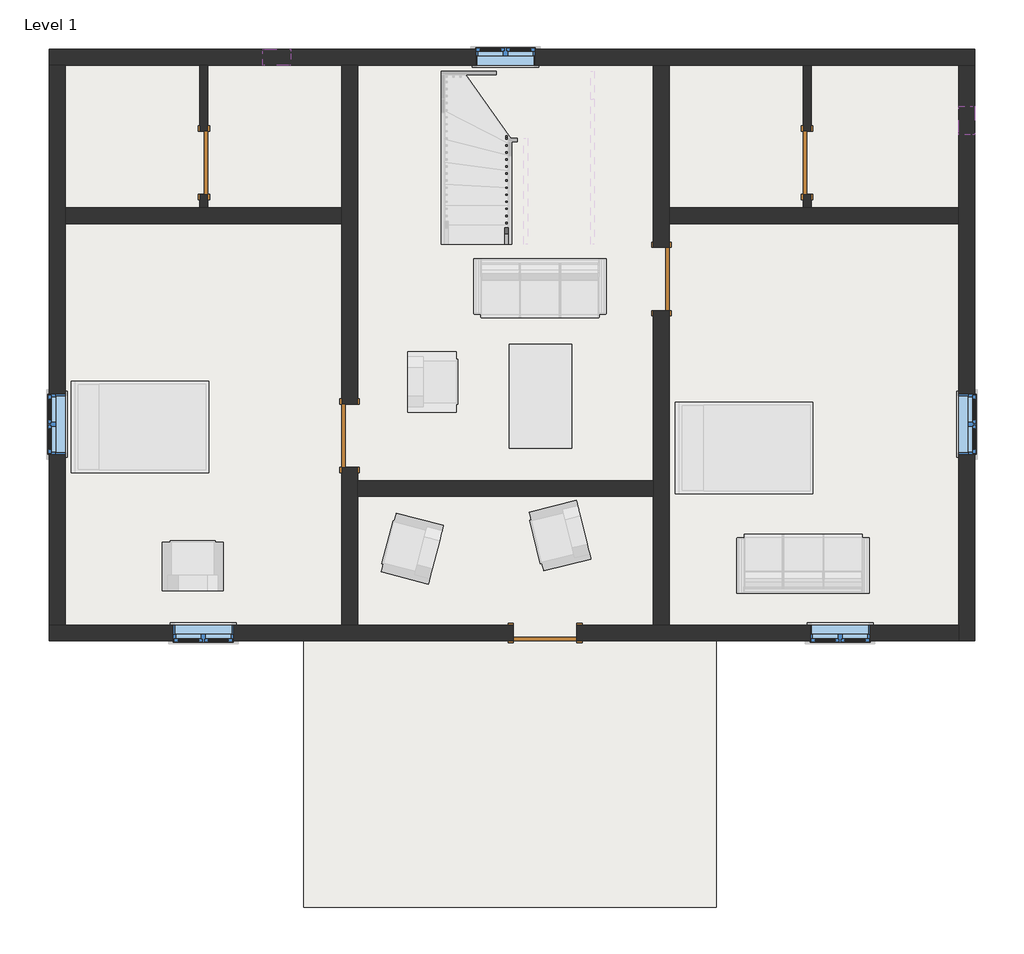
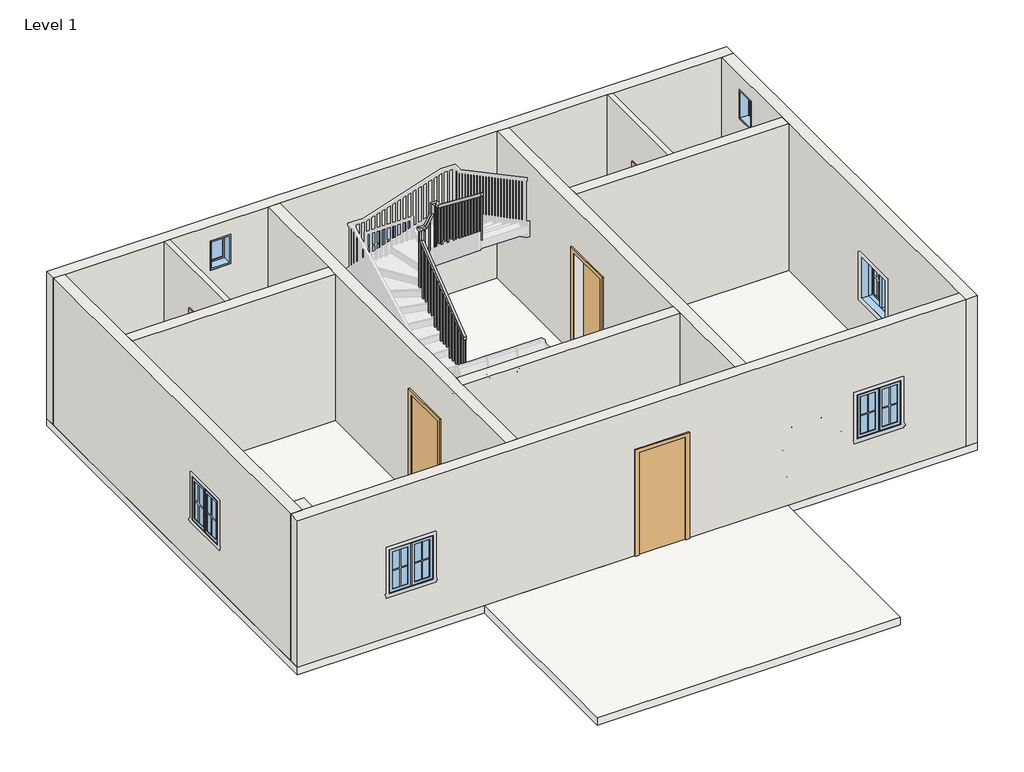
# One storey, part 1 of 2: 11 walls, 7 windows, 5 doors, 2 slabs, 1 railing.
"""IFC4 building model written with IfcOpenShell, lengths in millimetres."""

from ifc_helpers import new_model, si_unit, frame, origin, origin_with_axes, place, context, project, spatial, polyline, outline, extrude, faceted_brep, transform, mapped, element, save
from components import door_e5f9f3c4, door_a90ba1ad, door_305aa2a5, door_0ca8825f, window_aa618e30, window_339605e1

model = new_model("IFC4")

# Units and contexts
model_context = context("Model", 3, world=origin())
ifc_project = project(units=[si_unit("LENGTHUNIT", "METRE", prefix="MILLI")], contexts=[model_context])

# Site, building, storey
site = spatial("IfcSite", under=ifc_project)
building = spatial("IfcBuilding", under=site)
storey = spatial("IfcBuildingStorey", under=building, Name="Level 1", Elevation=0.0)

# Doors
placement = place(None, origin())
door_shape = door_e5f9f3c4(model_context)
element("IfcDoor", 1, ObjectType="Single-Flush : 36\" x 84\"", at=placement, inside=storey, context=model_context, shape_type="MappedRepresentation", body=[
    mapped(door_shape, transform((-5102.9390964, 4820.103532, 0.0), x_axis=(0.0, -1.0, 0.0), y_axis=(1.0, 0.0, 0.0), z_axis=(0.0, 0.0, 1.0))),
])
door_2_shape = door_a90ba1ad(model_context)
element("IfcDoor", 2, ObjectType="Single-Flush : 36\" x 84\"", at=placement, inside=storey, context=model_context, shape_type="MappedRepresentation", body=[
    mapped(door_2_shape, transform((-3001.0890964, 883.103532, 0.0), x_axis=(0.0, -1.0, 0.0), y_axis=(1.0, 0.0, 0.0), z_axis=(0.0, 0.0, 1.0))),
])
element("IfcDoor", 3, ObjectType="Single-Flush : 36\" x 84\"", at=placement, inside=storey, context=model_context, shape_type="MappedRepresentation", body=[
    mapped(door_2_shape, transform((1494.7109036, 3143.703532, 0.0), x_axis=(0.0, 1.0, 0.0), y_axis=(-1.0, 0.0, 0.0), z_axis=(0.0, 0.0, 1.0))),
])
door_3_shape = door_305aa2a5(model_context)
element("IfcDoor", 4, ObjectType="Single-Flush : 36\" x 84\"", at=placement, inside=storey, context=model_context, shape_type="MappedRepresentation", body=[
    mapped(door_3_shape, transform((3596.5609036, 4820.103532, 0.0), x_axis=(0.0, -1.0, 0.0), y_axis=(1.0, 0.0, 0.0), z_axis=(0.0, 0.0, 1.0))),
])
door_4_shape = door_0ca8825f(model_context)
element("IfcDoor", 5, ObjectType="Single-Flush : 36\" x 84\"", at=placement, inside=storey, context=model_context, shape_type="MappedRepresentation", body=[
    mapped(door_4_shape, transform((-181.6890964, -1961.696468, 0.0), x_axis=(-1.0, 0.0, 0.0), y_axis=(0.0, -1.0, 0.0), z_axis=(0.0, 0.0, 1.0))),
])

# Railing
element("IfcRailing", 6, ObjectType="Handrail - Rectangular", at=placement, inside=storey, context=model_context, shape_type="SolidModel", body=[
    faceted_brep([(-765.8890964, 3647.9718401, 1083.7333333), (-765.8890964, 3647.9718401, 1019.4000346), (-715.0890964, 3647.9718401, 1019.4000346), (-715.0890964, 3647.9718401, 1083.7333333), (-765.8890964, 5099.503532, 2211.6191036), (-765.8890964, 5150.303532, 2186.7590024), (-715.0890964, 5150.303532, 2186.7590024), (-715.0890964, 5099.503532, 2211.6191036), (-765.8890964, 5099.503532, 2414.6281882), (-765.8890964, 5150.303532, 2363.8281882), (-715.0890964, 5150.303532, 2363.8281882), (-715.0890964, 5099.503532, 2414.6281882), (-765.8890964, 5226.503532, 2414.6281882), (-765.8890964, 5226.503532, 2363.8281882), (-715.0890964, 5175.703532, 2363.8281882), (-715.0890964, 5175.703532, 2414.6281882), (-638.8890964, 5226.503532, 2414.6281882), (-609.7677625, 5226.503532, 2363.8281882), (-609.7677625, 5175.703532, 2363.8281882), (-638.8890964, 5175.703532, 2414.6281882), (-511.8890964, 5226.503532, 2631.5051451), (-461.0890964, 5226.503532, 2617.7256424), (-461.0890964, 5175.703532, 2617.7256424), (-511.8890964, 5175.703532, 2631.5051451), (-511.8890964, 5226.503532, 2834.5142297), (-461.0890964, 5226.503532, 2783.7142297), (-461.0890964, 5175.703532, 2783.7142297), (-511.8890964, 5175.703532, 2834.5142297), (-384.8890964, 5226.503532, 2834.5142297), (-384.8890964, 5226.503532, 2783.7142297), (-435.6890964, 5175.703532, 2783.7142297), (-435.6890964, 5175.703532, 2834.5142297), (-384.8890964, 5099.503532, 2834.5142297), (-384.8890964, 5082.086864, 2783.7142297), (-435.6890964, 5082.086864, 2783.7142297), (-435.6890964, 5099.503532, 2834.5142297), (-384.8890964, 3647.9718401, 3962.4), (-435.6890964, 3647.9718401, 3962.4), (-435.6890964, 3647.9718401, 3898.0667013), (-384.8890964, 3647.9718401, 3898.0667013)], [[[0, 1, 2, 3]], [[1, 0, 4, 5]], [[2, 1, 5, 6]], [[3, 2, 6, 7]], [[0, 3, 7, 4]], [[5, 4, 8, 9]], [[6, 5, 9, 10]], [[7, 6, 10, 11]], [[4, 7, 11, 8]], [[9, 8, 12, 13]], [[10, 9, 13, 14]], [[11, 10, 14, 15]], [[8, 11, 15, 12]], [[13, 12, 16, 17]], [[14, 13, 17, 18]], [[15, 14, 18, 19]], [[12, 15, 19, 16]], [[17, 16, 20, 21]], [[18, 17, 21, 22]], [[19, 18, 22, 23]], [[16, 19, 23, 20]], [[21, 20, 24, 25]], [[22, 21, 25, 26]], [[23, 22, 26, 27]], [[20, 23, 27, 24]], [[25, 24, 28, 29]], [[26, 25, 29, 30]], [[27, 26, 30, 31]], [[24, 27, 31, 28]], [[29, 28, 32, 33]], [[30, 29, 33, 34]], [[31, 30, 34, 35]], [[28, 31, 35, 32]], [[36, 37, 38, 39]], [[33, 32, 36, 39]], [[34, 33, 39, 38]], [[35, 34, 38, 37]], [[32, 35, 37, 36]]]),
    extrude(outline(polyline([(3667.578532, 3882.8316852), (3686.628532, 3868.0292361), (3686.628532, 2878.6666667), (3667.578532, 2878.6666667), (3667.578532, 3882.8316852)])), frame((-419.8140964, 0.0, 0.0), z_axis=(1.0, 0.0, 0.0), x_axis=(0.0, 1.0, 0.0)), (0.0, 0.0, 1.0), 19.05),
    extrude(outline(polyline([(3769.178532, 3803.8852902), (3788.228532, 3789.0828411), (3788.228532, 2878.6666667), (3769.178532, 2878.6666667), (3769.178532, 3803.8852902)])), frame((-419.8140964, 0.0, 0.0), z_axis=(1.0, 0.0, 0.0), x_axis=(0.0, 1.0, 0.0)), (0.0, 0.0, 1.0), 19.05),
    extrude(outline(polyline([(3870.778532, 3724.9388952), (3889.828532, 3710.1364462), (3889.828532, 2878.6666667), (3870.778532, 2878.6666667), (3870.778532, 3724.9388952)])), frame((-419.8140964, 0.0, 0.0), z_axis=(1.0, 0.0, 0.0), x_axis=(0.0, 1.0, 0.0)), (0.0, 0.0, 1.0), 19.05),
    extrude(outline(polyline([(3972.378532, 3645.9925003), (3991.428532, 3631.1900512), (3991.428532, 2709.3333333), (3972.378532, 2709.3333333), (3972.378532, 3645.9925003)])), frame((-419.8140964, 0.0, 0.0), z_axis=(1.0, 0.0, 0.0), x_axis=(0.0, 1.0, 0.0)), (0.0, 0.0, 1.0), 19.05),
    extrude(outline(polyline([(4073.978532, 3567.0461053), (4093.028532, 3552.2436562), (4093.028532, 2709.3333333), (4073.978532, 2709.3333333), (4073.978532, 3567.0461053)])), frame((-419.8140964, 0.0, 0.0), z_axis=(1.0, 0.0, 0.0), x_axis=(0.0, 1.0, 0.0)), (0.0, 0.0, 1.0), 19.05),
    extrude(outline(polyline([(4175.578532, 3488.0997103), (4194.628532, 3473.2972613), (4194.628532, 2709.3333333), (4175.578532, 2709.3333333), (4175.578532, 3488.0997103)])), frame((-419.8140964, 0.0, 0.0), z_axis=(1.0, 0.0, 0.0), x_axis=(0.0, 1.0, 0.0)), (0.0, 0.0, 1.0), 19.05),
    extrude(outline(polyline([(4277.178532, 3409.1533154), (4296.228532, 3394.3508663), (4296.228532, 2540.0), (4277.178532, 2540.0), (4277.178532, 3409.1533154)])), frame((-419.8140964, 0.0, 0.0), z_axis=(1.0, 0.0, 0.0), x_axis=(0.0, 1.0, 0.0)), (0.0, 0.0, 1.0), 19.05),
    extrude(outline(polyline([(4378.778532, 3330.2069204), (4397.828532, 3315.4044713), (4397.828532, 2540.0), (4378.778532, 2540.0), (4378.778532, 3330.2069204)])), frame((-419.8140964, 0.0, 0.0), z_axis=(1.0, 0.0, 0.0), x_axis=(0.0, 1.0, 0.0)), (0.0, 0.0, 1.0), 19.05),
    extrude(outline(polyline([(4480.378532, 3251.2605254), (4499.428532, 3236.4580764), (4499.428532, 2370.6666667), (4480.378532, 2370.6666667), (4480.378532, 3251.2605254)])), frame((-419.8140964, 0.0, 0.0), z_axis=(1.0, 0.0, 0.0), x_axis=(0.0, 1.0, 0.0)), (0.0, 0.0, 1.0), 19.05),
    extrude(outline(polyline([(4581.978532, 3172.3141304), (4601.028532, 3157.5116814), (4601.028532, 2370.6666667), (4581.978532, 2370.6666667), (4581.978532, 3172.3141304)])), frame((-419.8140964, 0.0, 0.0), z_axis=(1.0, 0.0, 0.0), x_axis=(0.0, 1.0, 0.0)), (0.0, 0.0, 1.0), 19.05),
    extrude(outline(polyline([(4683.578532, 3093.3677355), (4702.628532, 3078.5652864), (4702.628532, 2370.6666667), (4683.578532, 2370.6666667), (4683.578532, 3093.3677355)])), frame((-419.8140964, 0.0, 0.0), z_axis=(1.0, 0.0, 0.0), x_axis=(0.0, 1.0, 0.0)), (0.0, 0.0, 1.0), 19.05),
    extrude(outline(polyline([(4785.178532, 3014.4213405), (4804.228532, 2999.6188914), (4804.228532, 2201.3333333), (4785.178532, 2201.3333333), (4785.178532, 3014.4213405)])), frame((-419.8140964, 0.0, 0.0), z_axis=(1.0, 0.0, 0.0), x_axis=(0.0, 1.0, 0.0)), (0.0, 0.0, 1.0), 19.05),
    extrude(outline(polyline([(4886.778532, 2935.4749455), (4905.828532, 2920.6724965), (4905.828532, 2201.3333333), (4886.778532, 2201.3333333), (4886.778532, 2935.4749455)])), frame((-419.8140964, 0.0, 0.0), z_axis=(1.0, 0.0, 0.0), x_axis=(0.0, 1.0, 0.0)), (0.0, 0.0, 1.0), 19.05),
    extrude(outline(polyline([(4988.378532, 2856.5285506), (5007.428532, 2841.7261015), (5007.428532, 2032.0), (4988.378532, 2032.0), (4988.378532, 2856.5285506)])), frame((-419.8140964, 0.0, 0.0), z_axis=(1.0, 0.0, 0.0), x_axis=(0.0, 1.0, 0.0)), (0.0, 0.0, 1.0), 19.05),
    extrude(outline(polyline([(5089.978532, 2777.5821556), (5109.028532, 2762.7797065), (5109.028532, 2032.0), (5089.978532, 2032.0), (5089.978532, 2777.5821556)])), frame((-419.8140964, 0.0, 0.0), z_axis=(1.0, 0.0, 0.0), x_axis=(0.0, 1.0, 0.0)), (0.0, 0.0, 1.0), 19.05),
    extrude(outline(polyline([(-445.2140964, 5191.578532), (-445.2140964, 5210.628532), (-426.1640964, 5210.628532), (-426.1640964, 5191.578532), (-445.2140964, 5191.578532)])), frame((0.0, 0.0, 1693.3333333), z_axis=(0.0, 0.0, 1.0), x_axis=(1.0, 0.0, 0.0)), (0.0, 0.0, 1.0), 1090.3808964),
    extrude(outline(polyline([(2503.86524, -527.7640964), (2471.3336964, -546.8140964), (1524.0, -546.8140964), (1524.0, -527.7640964), (2503.86524, -527.7640964)])), frame((0.0, 5191.578532, 0.0), z_axis=(0.0, 1.0, 0.0), x_axis=(0.0, 0.0, 1.0)), (0.0, 0.0, 1.0), 19.05),
    extrude(outline(polyline([(2330.3636744, -629.3640964), (2297.8321309, -648.4140964), (1354.6666667, -648.4140964), (1354.6666667, -629.3640964), (2330.3636744, -629.3640964)])), frame((0.0, 5191.578532, 0.0), z_axis=(0.0, 1.0, 0.0), x_axis=(0.0, 0.0, 1.0)), (0.0, 0.0, 1.0), 19.05),
    extrude(outline(polyline([(-730.9640964, 5162.4468401), (-750.0140964, 5162.4468401), (-750.0140964, 5181.4968401), (-730.9640964, 5181.4968401), (-730.9640964, 5162.4468401)])), frame((0.0, 0.0, 1185.3333333), z_axis=(0.0, 0.0, 1.0), x_axis=(1.0, 0.0, 0.0)), (0.0, 0.0, 1.0), 1178.4948549),
    extrude(outline(polyline([(5060.8468401, 2117.2483397), (5079.8968401, 2132.0507888), (5079.8968401, 1016.0), (5060.8468401, 1016.0), (5060.8468401, 2117.2483397)])), frame((-750.0140964, 0.0, 0.0), z_axis=(1.0, 0.0, 0.0), x_axis=(0.0, 1.0, 0.0)), (0.0, 0.0, 1.0), 19.05),
    extrude(outline(polyline([(4959.2468401, 2038.3019447), (4978.2968401, 2053.1043938), (4978.2968401, 1016.0), (4959.2468401, 1016.0), (4959.2468401, 2038.3019447)])), frame((-750.0140964, 0.0, 0.0), z_axis=(1.0, 0.0, 0.0), x_axis=(0.0, 1.0, 0.0)), (0.0, 0.0, 1.0), 19.05),
    extrude(outline(polyline([(4857.6468401, 1959.3555498), (4876.6968401, 1974.1579988), (4876.6968401, 846.6666667), (4857.6468401, 846.6666667), (4857.6468401, 1959.3555498)])), frame((-750.0140964, 0.0, 0.0), z_axis=(1.0, 0.0, 0.0), x_axis=(0.0, 1.0, 0.0)), (0.0, 0.0, 1.0), 19.05),
    extrude(outline(polyline([(4756.0468401, 1880.4091548), (4775.0968401, 1895.2116039), (4775.0968401, 846.6666667), (4756.0468401, 846.6666667), (4756.0468401, 1880.4091548)])), frame((-750.0140964, 0.0, 0.0), z_axis=(1.0, 0.0, 0.0), x_axis=(0.0, 1.0, 0.0)), (0.0, 0.0, 1.0), 19.05),
    extrude(outline(polyline([(4654.4468401, 1801.4627598), (4673.4968401, 1816.2652089), (4673.4968401, 677.3333333), (4654.4468401, 677.3333333), (4654.4468401, 1801.4627598)])), frame((-750.0140964, 0.0, 0.0), z_axis=(1.0, 0.0, 0.0), x_axis=(0.0, 1.0, 0.0)), (0.0, 0.0, 1.0), 19.05),
    extrude(outline(polyline([(4552.8468401, 1722.5163649), (4571.8968401, 1737.3188139), (4571.8968401, 677.3333333), (4552.8468401, 677.3333333), (4552.8468401, 1722.5163649)])), frame((-750.0140964, 0.0, 0.0), z_axis=(1.0, 0.0, 0.0), x_axis=(0.0, 1.0, 0.0)), (0.0, 0.0, 1.0), 19.05),
    extrude(outline(polyline([(4451.2468401, 1643.5699699), (4470.2968401, 1658.3724189), (4470.2968401, 508.0), (4451.2468401, 508.0), (4451.2468401, 1643.5699699)])), frame((-750.0140964, 0.0, 0.0), z_axis=(1.0, 0.0, 0.0), x_axis=(0.0, 1.0, 0.0)), (0.0, 0.0, 1.0), 19.05),
    extrude(outline(polyline([(4349.6468401, 1564.6235749), (4368.6968401, 1579.426024), (4368.6968401, 508.0), (4349.6468401, 508.0), (4349.6468401, 1564.6235749)])), frame((-750.0140964, 0.0, 0.0), z_axis=(1.0, 0.0, 0.0), x_axis=(0.0, 1.0, 0.0)), (0.0, 0.0, 1.0), 19.05),
    extrude(outline(polyline([(4248.0468401, 1485.6771799), (4267.0968401, 1500.479629), (4267.0968401, 508.0), (4248.0468401, 508.0), (4248.0468401, 1485.6771799)])), frame((-750.0140964, 0.0, 0.0), z_axis=(1.0, 0.0, 0.0), x_axis=(0.0, 1.0, 0.0)), (0.0, 0.0, 1.0), 19.05),
    extrude(outline(polyline([(4146.4468401, 1406.730785), (4165.4968401, 1421.533234), (4165.4968401, 338.6666667), (4146.4468401, 338.6666667), (4146.4468401, 1406.730785)])), frame((-750.0140964, 0.0, 0.0), z_axis=(1.0, 0.0, 0.0), x_axis=(0.0, 1.0, 0.0)), (0.0, 0.0, 1.0), 19.05),
    extrude(outline(polyline([(4044.8468401, 1327.78439), (4063.8968401, 1342.5868391), (4063.8968401, 338.6666667), (4044.8468401, 338.6666667), (4044.8468401, 1327.78439)])), frame((-750.0140964, 0.0, 0.0), z_axis=(1.0, 0.0, 0.0), x_axis=(0.0, 1.0, 0.0)), (0.0, 0.0, 1.0), 19.05),
    extrude(outline(polyline([(3943.2468401, 1248.837995), (3962.2968401, 1263.6404441), (3962.2968401, 338.6666667), (3943.2468401, 338.6666667), (3943.2468401, 1248.837995)])), frame((-750.0140964, 0.0, 0.0), z_axis=(1.0, 0.0, 0.0), x_axis=(0.0, 1.0, 0.0)), (0.0, 0.0, 1.0), 19.05),
    extrude(outline(polyline([(3841.6468401, 1169.8916001), (3860.6968401, 1184.6940491), (3860.6968401, 169.3333333), (3841.6468401, 169.3333333), (3841.6468401, 1169.8916001)])), frame((-750.0140964, 0.0, 0.0), z_axis=(1.0, 0.0, 0.0), x_axis=(0.0, 1.0, 0.0)), (0.0, 0.0, 1.0), 19.05),
    extrude(outline(polyline([(3740.0468401, 1090.9452051), (3759.0968401, 1105.7476541), (3759.0968401, 169.3333333), (3740.0468401, 169.3333333), (3740.0468401, 1090.9452051)])), frame((-750.0140964, 0.0, 0.0), z_axis=(1.0, 0.0, 0.0), x_axis=(0.0, 1.0, 0.0)), (0.0, 0.0, 1.0), 19.05),
    extrude(outline(polyline([(-419.8140964, 5191.578532), (-419.8140964, 5210.628532), (-400.7640964, 5210.628532), (-400.7640964, 5191.578532), (-419.8140964, 5191.578532)])), frame((0.0, 0.0, 1862.6666667), z_axis=(0.0, 0.0, 1.0), x_axis=(1.0, 0.0, 0.0)), (0.0, 0.0, 1.0), 921.0475631),
    extrude(outline(polyline([(-730.9640964, 5191.578532), (-750.0140964, 5191.578532), (-750.0140964, 5210.628532), (-730.9640964, 5210.628532), (-730.9640964, 5191.578532)])), frame((0.0, 0.0, 1185.3333333), z_axis=(0.0, 0.0, 1.0), x_axis=(1.0, 0.0, 0.0)), (0.0, 0.0, 1.0), 1178.4948549),
    extrude(outline(polyline([(3647.9718401, 3898.0667013), (3667.0218401, 3883.2642523), (3667.0218401, 2878.6666667), (3647.9718401, 2878.6666667), (3647.9718401, 3898.0667013)])), frame((-419.8140964, 0.0, 0.0), z_axis=(1.0, 0.0, 0.0), x_axis=(0.0, 1.0, 0.0)), (0.0, 0.0, 1.0), 19.05),
    extrude(outline(polyline([(3647.9718401, 1019.4000346), (3667.0218401, 1034.2024837), (3667.0218401, 169.3333333), (3647.9718401, 169.3333333), (3647.9718401, 1019.4000346)])), frame((-750.0140964, 0.0, 0.0), z_axis=(1.0, 0.0, 0.0), x_axis=(0.0, 1.0, 0.0)), (0.0, 0.0, 1.0), 19.05),
])

# Slabs
element("IfcSlab", 7, ObjectType="Generic - 12\"", at=placement, inside=storey, context=model_context, shape_type="SweptSolid", body=[
    extrude(outline(polyline([(6015.9109036, 6458.403532), (6015.9109036, -2075.996468), (-7334.9640964, -2075.996468), (-7334.9640964, 6458.403532), (6015.9109036, 6458.403532)])), frame((0.0, 0.0, -152.4), z_axis=(0.0, 0.0, 1.0), x_axis=(1.0, 0.0, 0.0)), (0.0, 0.0, 1.0), 152.4),
])
element("IfcSlab", 8, ObjectType="Generic - 12\"", at=placement, inside=storey, context=model_context, shape_type="SweptSolid", body=[
    extrude(outline(polyline([(2286.9448179, -2075.996468), (2286.9448179, -5916.2427923), (-3666.7326554, -5916.2427923), (-3666.7326554, -2075.996468), (2286.9448179, -2075.996468)])), frame((0.0, 0.0, -152.4), z_axis=(0.0, 0.0, 1.0), x_axis=(1.0, 0.0, 0.0)), (0.0, 0.0, 1.0), 152.4),
])

# Walls
element("IfcWall", 9, ObjectType="WALL4.5\"", at=placement, inside=storey, context=model_context, shape_type="SweptSolid", body=[
    extrude(outline(polyline([(4362.903532, 2133.6), (4362.903532, 0.0), (4172.403532, 0.0), (4172.403532, 3048.0), (6229.803532, 3048.0), (6229.803532, 0.0), (5277.303532, 0.0), (5277.303532, 2133.6), (4362.903532, 2133.6)])), frame((-5160.0890964, 0.0, 0.0), z_axis=(1.0, 0.0, 0.0), x_axis=(0.0, 1.0, 0.0)), (0.0, 0.0, 1.0), 114.3),
])
element("IfcWall", 10, ObjectType="WALL4.5\"", at=placement, inside=storey, context=model_context, shape_type="SweptSolid", body=[
    extrude(outline(polyline([(4362.903532, 2133.6), (4362.903532, 0.0), (4172.403532, 0.0), (4172.403532, 3048.0), (6229.803532, 3048.0), (6229.803532, 0.0), (5277.303532, 0.0), (5277.303532, 2133.6), (4362.903532, 2133.6)])), frame((3539.4109036, 0.0, 0.0), z_axis=(1.0, 0.0, 0.0), x_axis=(0.0, 1.0, 0.0)), (0.0, 0.0, 1.0), 114.3),
])
element("IfcWall", 11, ObjectType="WALL9\"", at=placement, inside=storey, context=model_context, shape_type="Brep", body=[
    faceted_brep([(-7334.9640964, 6229.803532, 0.0), (-7106.3640964, 6229.803532, 0.0), (-5160.0890964, 6229.803532, 0.0), (-5045.7890964, 6229.803532, 0.0), (-3115.3890964, 6229.803532, 0.0), (-2886.7890964, 6229.803532, 0.0), (1380.4109036, 6229.803532, 0.0), (1609.0109036, 6229.803532, 0.0), (3539.4109036, 6229.803532, 0.0), (3653.7109036, 6229.803532, 0.0), (5787.3109036, 6229.803532, 0.0), (6015.9109036, 6229.803532, 0.0), (6015.9109036, 6229.803532, 3048.0), (5787.3109036, 6229.803532, 3048.0), (3653.7109036, 6229.803532, 3048.0), (3539.4109036, 6229.803532, 3048.0), (1609.0109036, 6229.803532, 3048.0), (1380.4109036, 6229.803532, 3048.0), (-2886.7890964, 6229.803532, 3048.0), (-3115.3890964, 6229.803532, 3048.0), (-5045.7890964, 6229.803532, 3048.0), (-5160.0890964, 6229.803532, 3048.0), (-7106.3640964, 6229.803532, 3048.0), (-7334.9640964, 6229.803532, 3048.0), (-3848.8140964, 6229.803532, 2743.2), (-3848.8140964, 6229.803532, 2133.6), (-4255.2140964, 6229.803532, 2133.6), (-4255.2140964, 6229.803532, 2743.2), (-321.3890964, 6229.803532, 1828.8), (-321.3890964, 6229.803532, 914.4), (-1184.9890964, 6229.803532, 914.4), (-1184.9890964, 6229.803532, 1828.8), (-7334.9640964, 6458.403532, 0.0), (-7334.9640964, 6458.403532, 3048.0), (6015.9109036, 6458.403532, 3048.0), (6015.9109036, 6458.403532, 0.0), (-3848.8140964, 6458.403532, 2743.2), (-4255.2140964, 6458.403532, 2743.2), (-4255.2140964, 6458.403532, 2133.6), (-3848.8140964, 6458.403532, 2133.6), (-321.3890964, 6458.403532, 1828.8), (-1184.9890964, 6458.403532, 1828.8), (-1184.9890964, 6458.403532, 914.4), (-321.3890964, 6458.403532, 914.4)], [[[0, 1, 2, 3, 4, 5, 6, 7, 8, 9, 10, 11, 12, 13, 14, 15, 16, 17, 18, 19, 20, 21, 22, 23], [24, 25, 26, 27], [28, 29, 30, 31]], [[32, 33, 34, 35], [36, 37, 38, 39], [40, 41, 42, 43]], [[11, 10, 9, 8, 7, 6, 5, 4, 3, 2, 1, 0, 32, 35]], [[12, 11, 35, 34]], [[0, 23, 33, 32]], [[25, 24, 36, 39]], [[26, 25, 39, 38]], [[27, 26, 38, 37]], [[24, 27, 37, 36]], [[29, 28, 40, 43]], [[30, 29, 43, 42]], [[31, 30, 42, 41]], [[28, 31, 41, 40]], [[23, 22, 21, 20, 19, 18, 17, 16, 15, 14, 13, 12, 34, 33]]]),
])
element("IfcWall", 12, ObjectType="WALL9\"", at=placement, inside=storey, context=model_context, shape_type="Brep", body=[
    faceted_brep([(5787.3109036, 6229.803532, 0.0), (5787.3109036, 4172.403532, 0.0), (5787.3109036, 3943.803532, 0.0), (5787.3109036, -1847.396468, 0.0), (5787.3109036, -2075.996468, 0.0), (5787.3109036, -2075.996468, 3048.0), (5787.3109036, -1847.396468, 3048.0), (5787.3109036, 3943.803532, 3048.0), (5787.3109036, 4172.403532, 3048.0), (5787.3109036, 6229.803532, 3048.0), (5787.3109036, 5226.503532, 2743.2), (5787.3109036, 5226.503532, 2133.6), (5787.3109036, 5632.903532, 2133.6), (5787.3109036, 5632.903532, 2743.2), (5787.3109036, 616.403532, 1828.8), (5787.3109036, 616.403532, 914.4), (5787.3109036, 1480.003532, 914.4), (5787.3109036, 1480.003532, 1828.8), (6015.9109036, 6229.803532, 0.0), (6015.9109036, 6229.803532, 3048.0), (6015.9109036, -2075.996468, 3048.0), (6015.9109036, -2075.996468, 0.0), (6015.9109036, 5226.503532, 2743.2), (6015.9109036, 5632.903532, 2743.2), (6015.9109036, 5632.903532, 2133.6), (6015.9109036, 5226.503532, 2133.6), (6015.9109036, 616.403532, 1828.8), (6015.9109036, 1480.003532, 1828.8), (6015.9109036, 1480.003532, 914.4), (6015.9109036, 616.403532, 914.4)], [[[0, 1, 2, 3, 4, 5, 6, 7, 8, 9], [10, 11, 12, 13], [14, 15, 16, 17]], [[18, 19, 20, 21], [22, 23, 24, 25], [26, 27, 28, 29]], [[4, 3, 2, 1, 0, 18, 21]], [[0, 9, 19, 18]], [[5, 4, 21, 20]], [[11, 10, 22, 25]], [[12, 11, 25, 24]], [[13, 12, 24, 23]], [[10, 13, 23, 22]], [[15, 14, 26, 29]], [[16, 15, 29, 28]], [[17, 16, 28, 27]], [[14, 17, 27, 26]], [[9, 8, 7, 6, 5, 20, 19]]]),
])
element("IfcWall", 13, ObjectType="WALL9\"", at=placement, inside=storey, context=model_context, shape_type="Brep", body=[
    faceted_brep([(-638.8890964, -1847.396468, 2133.6), (-638.8890964, -1847.396468, 0.0), (-2886.7890964, -1847.396468, 0.0), (-3115.3890964, -1847.396468, 0.0), (-7106.3640964, -1847.396468, 0.0), (-7334.9640964, -1847.396468, 0.0), (-7334.9640964, -1847.396468, 3048.0), (-7106.3640964, -1847.396468, 3048.0), (-3115.3890964, -1847.396468, 3048.0), (-2886.7890964, -1847.396468, 3048.0), (1380.4109036, -1847.396468, 3048.0), (1609.0109036, -1847.396468, 3048.0), (5787.3109036, -1847.396468, 3048.0), (5787.3109036, -1847.396468, 0.0), (1609.0109036, -1847.396468, 0.0), (1380.4109036, -1847.396468, 0.0), (275.5109036, -1847.396468, 0.0), (275.5109036, -1847.396468, 2133.6), (-5542.6765964, -1847.396468, 1828.8), (-5542.6765964, -1847.396468, 914.4), (-4679.0765964, -1847.396468, 914.4), (-4679.0765964, -1847.396468, 1828.8), (3641.0109036, -1847.396468, 1828.8), (3641.0109036, -1847.396468, 914.4), (4504.6109036, -1847.396468, 914.4), (4504.6109036, -1847.396468, 1828.8), (-7334.9640964, -2075.996468, 0.0), (-638.8890964, -2075.996468, 0.0), (-638.8890964, -2075.996468, 2133.6), (275.5109036, -2075.996468, 2133.6), (275.5109036, -2075.996468, 0.0), (5787.3109036, -2075.996468, 0.0), (5787.3109036, -2075.996468, 3048.0), (-7334.9640964, -2075.996468, 3048.0), (-5542.6765964, -2075.996468, 1828.8), (-4679.0765964, -2075.996468, 1828.8), (-4679.0765964, -2075.996468, 914.4), (-5542.6765964, -2075.996468, 914.4), (3641.0109036, -2075.996468, 1828.8), (4504.6109036, -2075.996468, 1828.8), (4504.6109036, -2075.996468, 914.4), (3641.0109036, -2075.996468, 914.4)], [[[0, 1, 2, 3, 4, 5, 6, 7, 8, 9, 10, 11, 12, 13, 14, 15, 16, 17], [18, 19, 20, 21], [22, 23, 24, 25]], [[26, 27, 28, 29, 30, 31, 32, 33], [34, 35, 36, 37], [38, 39, 40, 41]], [[5, 4, 3, 2, 1, 27, 26]], [[16, 15, 14, 13, 31, 30]], [[13, 12, 32, 31]], [[6, 5, 26, 33]], [[19, 18, 34, 37]], [[20, 19, 37, 36]], [[21, 20, 36, 35]], [[18, 21, 35, 34]], [[23, 22, 38, 41]], [[24, 23, 41, 40]], [[25, 24, 40, 39]], [[22, 25, 39, 38]], [[12, 11, 10, 9, 8, 7, 6, 33, 32]], [[28, 27, 1, 0]], [[29, 28, 0, 17]], [[30, 29, 17, 16]]]),
])
element("IfcWall", 14, ObjectType="WALL9\"", at=placement, inside=storey, context=model_context, shape_type="Brep", body=[
    faceted_brep([(-7106.3640964, -1847.396468, 0.0), (-7106.3640964, 3943.803532, 0.0), (-7106.3640964, 4172.403532, 0.0), (-7106.3640964, 6229.803532, 0.0), (-7106.3640964, 6229.803532, 3048.0), (-7106.3640964, 4172.403532, 3048.0), (-7106.3640964, 3943.803532, 3048.0), (-7106.3640964, -1847.396468, 3048.0), (-7106.3640964, 1480.003532, 1828.8), (-7106.3640964, 1480.003532, 914.4), (-7106.3640964, 616.403532, 914.4), (-7106.3640964, 616.403532, 1828.8), (-7334.9640964, -1847.396468, 0.0), (-7334.9640964, -1847.396468, 3048.0), (-7334.9640964, 6229.803532, 3048.0), (-7334.9640964, 6229.803532, 0.0), (-7334.9640964, 1480.003532, 1828.8), (-7334.9640964, 616.403532, 1828.8), (-7334.9640964, 616.403532, 914.4), (-7334.9640964, 1480.003532, 914.4)], [[[0, 1, 2, 3, 4, 5, 6, 7], [8, 9, 10, 11]], [[12, 13, 14, 15], [16, 17, 18, 19]], [[3, 2, 1, 0, 12, 15]], [[0, 7, 13, 12]], [[4, 3, 15, 14]], [[9, 8, 16, 19]], [[10, 9, 19, 18]], [[11, 10, 18, 17]], [[8, 11, 17, 16]], [[7, 6, 5, 4, 14, 13]]]),
])
element("IfcWall", 15, ObjectType="WALL9\"", at=placement, inside=storey, context=model_context, shape_type="Brep", body=[
    faceted_brep([(-3115.3890964, 425.903532, 2133.6), (-3115.3890964, 425.903532, 0.0), (-3115.3890964, -1847.396468, 0.0), (-3115.3890964, -1847.396468, 3048.0), (-3115.3890964, 3943.803532, 3048.0), (-3115.3890964, 4172.403532, 3048.0), (-3115.3890964, 6229.803532, 3048.0), (-3115.3890964, 6229.803532, 0.0), (-3115.3890964, 4172.403532, 0.0), (-3115.3890964, 3943.803532, 0.0), (-3115.3890964, 1340.303532, 0.0), (-3115.3890964, 1340.303532, 2133.6), (-2886.7890964, -1847.396468, 0.0), (-2886.7890964, 6.803532, 0.0), (-2886.7890964, 235.403532, 0.0), (-2886.7890964, 425.903532, 0.0), (-2886.7890964, 425.903532, 2133.6), (-2886.7890964, 1340.303532, 2133.6), (-2886.7890964, 1340.303532, 0.0), (-2886.7890964, 6229.803532, 0.0), (-2886.7890964, 6229.803532, 3048.0), (-2886.7890964, 235.403532, 3048.0), (-2886.7890964, 6.803532, 3048.0), (-2886.7890964, -1847.396468, 3048.0)], [[[0, 1, 2, 3, 4, 5, 6, 7, 8, 9, 10, 11]], [[12, 13, 14, 15, 16, 17, 18, 19, 20, 21, 22, 23]], [[2, 1, 15, 14, 13, 12]], [[10, 9, 8, 7, 19, 18]], [[7, 6, 20, 19]], [[3, 2, 12, 23]], [[16, 15, 1, 0]], [[17, 16, 0, 11]], [[18, 17, 11, 10]], [[6, 5, 4, 3, 23, 22, 21, 20]]]),
])
element("IfcWall", 16, ObjectType="WALL9\"", at=placement, inside=storey, context=model_context, shape_type="SweptSolid", body=[
    extrude(outline(polyline([(1380.4109036, 6.803532), (-2886.7890964, 6.803532), (-2886.7890964, 235.403532), (1380.4109036, 235.403532), (1380.4109036, 6.803532)])), origin_with_axes(), (0.0, 0.0, 1.0), 3048.0),
])
element("IfcWall", 17, ObjectType="WALL9\"", at=placement, inside=storey, context=model_context, shape_type="Brep", body=[
    faceted_brep([(1609.0109036, 3600.903532, 2133.6), (1609.0109036, 3600.903532, 0.0), (1609.0109036, 3943.803532, 0.0), (1609.0109036, 4172.403532, 0.0), (1609.0109036, 6229.803532, 0.0), (1609.0109036, 6229.803532, 3048.0), (1609.0109036, 4172.403532, 3048.0), (1609.0109036, 3943.803532, 3048.0), (1609.0109036, -1847.396468, 3048.0), (1609.0109036, -1847.396468, 0.0), (1609.0109036, 2686.503532, 0.0), (1609.0109036, 2686.503532, 2133.6), (1380.4109036, 6229.803532, 0.0), (1380.4109036, 3600.903532, 0.0), (1380.4109036, 3600.903532, 2133.6), (1380.4109036, 2686.503532, 2133.6), (1380.4109036, 2686.503532, 0.0), (1380.4109036, 235.403532, 0.0), (1380.4109036, 6.803532, 0.0), (1380.4109036, -1847.396468, 0.0), (1380.4109036, -1847.396468, 3048.0), (1380.4109036, 6.803532, 3048.0), (1380.4109036, 235.403532, 3048.0), (1380.4109036, 6229.803532, 3048.0)], [[[0, 1, 2, 3, 4, 5, 6, 7, 8, 9, 10, 11]], [[12, 13, 14, 15, 16, 17, 18, 19, 20, 21, 22, 23]], [[10, 9, 19, 18, 17, 16]], [[4, 3, 2, 1, 13, 12]], [[5, 4, 12, 23]], [[9, 8, 20, 19]], [[14, 13, 1, 0]], [[15, 14, 0, 11]], [[16, 15, 11, 10]], [[8, 7, 6, 5, 23, 22, 21, 20]]]),
])
element("IfcWall", 18, ObjectType="WALL9\"", at=placement, inside=storey, context=model_context, shape_type="Brep", body=[
    faceted_brep([(1609.0109036, 3943.803532, 0.0), (5787.3109036, 3943.803532, 0.0), (5787.3109036, 3943.803532, 3048.0), (1609.0109036, 3943.803532, 3048.0), (1609.0109036, 4172.403532, 0.0), (1609.0109036, 4172.403532, 3048.0), (3539.4109036, 4172.403532, 3048.0), (3653.7109036, 4172.403532, 3048.0), (5787.3109036, 4172.403532, 3048.0), (5787.3109036, 4172.403532, 0.0), (3653.7109036, 4172.403532, 0.0), (3539.4109036, 4172.403532, 0.0)], [[[0, 1, 2, 3]], [[4, 5, 6, 7, 8, 9, 10, 11]], [[1, 0, 4, 11, 10, 9]], [[2, 1, 9, 8]], [[0, 3, 5, 4]], [[3, 2, 8, 7, 6, 5]]]),
])
element("IfcWall", 19, ObjectType="WALL9\"", at=placement, inside=storey, context=model_context, shape_type="Brep", body=[
    faceted_brep([(-7106.3640964, 3943.803532, 0.0), (-3115.3890964, 3943.803532, 0.0), (-3115.3890964, 3943.803532, 3048.0), (-7106.3640964, 3943.803532, 3048.0), (-7106.3640964, 4172.403532, 0.0), (-7106.3640964, 4172.403532, 3048.0), (-5160.0890964, 4172.403532, 3048.0), (-5045.7890964, 4172.403532, 3048.0), (-3115.3890964, 4172.403532, 3048.0), (-3115.3890964, 4172.403532, 0.0), (-5045.7890964, 4172.403532, 0.0), (-5160.0890964, 4172.403532, 0.0)], [[[0, 1, 2, 3]], [[4, 5, 6, 7, 8, 9, 10, 11]], [[1, 0, 4, 11, 10, 9]], [[0, 3, 5, 4]], [[2, 1, 9, 8]], [[3, 2, 8, 7, 6, 5]]]),
])

# Windows
window_shape = window_aa618e30(model_context)
element("IfcWindow", 20, ObjectType="Fixed : 16\" x 24\"", at=placement, inside=storey, context=model_context, shape_type="MappedRepresentation", body=[
    mapped(window_shape, transform((-4013.9140964, 6344.103532, 1219.2), x_axis=(1.0, 0.0, 0.0), y_axis=(0.0, 1.0, 0.0), z_axis=(0.0, 0.0, 1.0))),
])
element("IfcWindow", 21, ObjectType="Fixed : 16\" x 24\"", at=placement, inside=storey, context=model_context, shape_type="MappedRepresentation", body=[
    mapped(window_shape, transform((5901.6109036, 5391.603532, 1219.2), x_axis=(0.0, -1.0, 0.0), y_axis=(1.0, 0.0, 0.0), z_axis=(0.0, 0.0, 1.0))),
])
window_2_shape = window_339605e1(model_context)
element("IfcWindow", 22, ObjectType="Window-Casement-Double : 34\" x 36\"", at=placement, inside=storey, context=model_context, shape_type="MappedRepresentation", body=[
    mapped(window_2_shape, transform((-7220.6640964, 1048.203532, 0.0), x_axis=(0.0, 1.0, 0.0), y_axis=(-1.0, 0.0, 0.0), z_axis=(0.0, 0.0, 1.0))),
])
element("IfcWindow", 23, ObjectType="Window-Casement-Double : 34\" x 36\"", at=placement, inside=storey, context=model_context, shape_type="MappedRepresentation", body=[
    mapped(window_2_shape, transform((5901.6109036, 1048.203532, 0.0), x_axis=(0.0, -1.0, 0.0), y_axis=(1.0, 0.0, 0.0), z_axis=(0.0, 0.0, 1.0))),
])
element("IfcWindow", 24, ObjectType="Window-Casement-Double : 34\" x 36\"", at=placement, inside=storey, context=model_context, shape_type="MappedRepresentation", body=[
    mapped(window_2_shape, transform((-753.1890964, 6344.103532, 0.0), x_axis=(1.0, 0.0, 0.0), y_axis=(0.0, 1.0, 0.0), z_axis=(0.0, 0.0, 1.0))),
])
element("IfcWindow", 25, ObjectType="Window-Casement-Double : 34\" x 36\"", at=placement, inside=storey, context=model_context, shape_type="MappedRepresentation", body=[
    mapped(window_2_shape, transform((-5110.8765964, -1961.696468, 0.0), x_axis=(-1.0, 0.0, 0.0), y_axis=(0.0, -1.0, 0.0), z_axis=(0.0, 0.0, 1.0))),
])
element("IfcWindow", 26, ObjectType="Window-Casement-Double : 34\" x 36\"", at=placement, inside=storey, context=model_context, shape_type="MappedRepresentation", body=[
    mapped(window_2_shape, transform((4072.8109036, -1961.696468, 0.0), x_axis=(-1.0, 0.0, 0.0), y_axis=(0.0, -1.0, 0.0), z_axis=(0.0, 0.0, 1.0))),
])

save(model, "model.ifc")

# Revit data of these elements
# Type "Single-Flush : 36\" x 84\""
#   Type Mark = "1"
#   Construction Type Id = "MDOOR"
#   Assembly Code = "C1020"
#   Analytic Construction = "Metal"
#   Thickness = 0' - 2"
#   Heat Transfer Coefficient (U) = 0.651978 BTU/(h·ft²·°F)
#   Height = 7' - 0"
#   Trim Projection Ext = 0' - 1"
#   Trim Projection Int = 0' - 1"
#   Trim Width = 0' - 3"
#   Width = 3' - 0"
#   Define Thermal Properties by = 1
#   Define Thermal Properties by = 1
#   Door Material = Door - Panel
#   Frame Material = Door - Frame
#   Visual Light Transmittance = 0
#   Solar Heat Gain Coefficient = 0
#   Function = (empty or 0)
#   Wall Closure = (empty or 0)
# Type "Handrail - Rectangular"
#   Assembly Code = "C2010400"
#   built-in parameter 1008612 = 0.0416667 (stored number, unit not read)
#   built-in parameter 1008611 = 0.0416667 (stored number, unit not read)
#   built-in parameter 1008609 = 0.333333 (stored number, unit not read)
#   built-in parameter 1008604 = 0.166667 (stored number, unit not read)
#   built-in parameter 1008603 = 0.166667 (stored number, unit not read)
#   Railing Height = 3' - 0"
#   built-in parameter 1008630 = 2
#   built-in parameter 1008610 = 2
#   built-in parameter 1008618 = Baluster - Square : 3/4"
# Type "Generic - 12\""
#   Assembly Code = "B1010"
#   Function = 0
#   Layers, outside or top first: 0' - 6" no material (function 1)
# Type "WALL4.5\""
#   Assembly Code = "B2010"
#   Layers, outside or top first: 0' - 4 1/2" no material (function 1)
# Type "WALL9\""
#   Assembly Code = "B2010"
#   Layers, outside or top first: 0' - 9" no material (function 1)
# Type "Fixed : 16\" x 24\""
#   Type Mark = "4"
#   Construction Type Id = "GSP4R"
#   Assembly Code = "B2020100"
#   Analytic Construction = "1/8 in Pilkington single glazing"
#   Visual Light Transmittance = 0.9
#   Solar Heat Gain Coefficient = 0.78
#   Heat Transfer Coefficient (U) = 0.6496 BTU/(h·ft²·°F)
#   Height = 2' - 0"
#   Default Sill Height = 3' - 0"
#   Width = 1' - 4"
#   Window Inset = 0' - 0 3/4"
#   Define Thermal Properties by = 1
#   Define Thermal Properties by = 1
#   Glass Pane Material = Glass
#   Sash Material = Sash
#   Wall Closure = (empty or 0)
# Type "Window-Casement-Double : 34\" x 36\""
#   Type Mark = "14"
#   Fire Rating = "0.5h"
#   Assembly Code = "B2020100"
#   Analytic Construction = "Double glazing - domestic"
#   Frame Extension [instance default] = 0' - 0 1/4"
#   Window Inset [instance default] = 0' - 0"
#   Wall Thickness [instance default] = 0' - 6"
#   Interior Wall Closure [instance default] = 0' - 2 1/4"
#   Half Width = 1' - 5"
#   Visual Light Transmittance = 0.81
#   Thermal Resistance (R) = 1.8146 (h·ft²·°F)/BTU
#   Solar Heat Gain Coefficient = 0.76
#   Rough Width = 2' - 10 1/2"
#   Rough Height = 3' - 0 1/2"
#   Height = 3' - 0"
#   Heat Transfer Coefficient (U) = 0.5511 BTU/(h·ft²·°F)
#   Exterior Wall Closure [instance default] = 0' - 1 1/4"
#   Extension Jamb [instance default] = 0' - 2 1/4"
#   Default Sill Height = 3' - 0"
#   Width = 2' - 10"
#   Define Thermal Properties by = 0
#   Muntin Visibility = yes
#   Interior Trim Visibility [instance default] = yes
#   Exterior Trim Visibility [instance default] = yes
#   Extension Jamb Visibility [instance default] = yes
#   Interior Trim Material = Wood - Stained
#   Muntin Pattern = Muntin Pattern_2x2 : Muntin Pattern_2x2
#   Interior Trim = Trim-Window-Interior-Flat : Picture Frame
#   Interior Frame Material = Wood - Stained
#   Glass Panel Material = Glass
#   Exterior Trim Material = Clad - White
#   Exterior Trim = Trim-Window-Exterior-Flat : with Sill
#   Exterior Frame Material = Clad - White
#   Wall Closure = (empty or 0)
# Elements 1, 2, 3, 4, 5 (IfcDoor, "Single-Flush : 36\" x 84\"")
#   Phase Created = New Construction
#   Materials on its faces: "Door - Frame", "Door - Panel"
# Element 6 (IfcRailing, "Handrail - Rectangular")
#   Phase Created = New Construction
# Elements 7, 8 (IfcSlab, "Generic - 12\"")
#   Height Offset From Level = 0' - 0"
#   Phase Created = New Construction
#   Materials on its faces: "Default Floor"
# Elements 9, 10 (IfcWall, "WALL4.5\"")
#   Top Offset = 0' - 0"
#   Base Offset = 0' - 0"
#   Unconnected Height = 10' - 0"
#   wall height = 10' - 0"
#   Phase Created = New Construction
#   Base Constraint = Level 1
#   Materials on its faces: "Default Wall"
# Elements 11, 12, 13, 14 (IfcWall, "WALL9\"")
#   Top Offset = 0' - 0"
#   Base Offset = 0' - 0"
#   Unconnected Height = 10' - 0"
#   wall height = 10' - 0"
#   Phase Created = New Construction
#   Base Constraint = Level 1
#   Materials on its faces: "Default Wall", "Wood Planks"
# Elements 15, 16, 17, 18, 19 (IfcWall, "WALL9\"")
#   Top Offset = 0' - 0"
#   Base Offset = 0' - 0"
#   Unconnected Height = 10' - 0"
#   wall height = 10' - 0"
#   Phase Created = New Construction
#   Base Constraint = Level 1
#   Materials on its faces: "Default Wall"
# Element 20 (IfcWindow, "Fixed : 16\" x 24\"")
#   Mark = "1"
#   Phase Created = New Construction
#   Materials on its faces: "Sash", "Glass"
# Element 21 (IfcWindow, "Fixed : 16\" x 24\"")
#   Mark = "2"
#   Phase Created = New Construction
#   Materials on its faces: "Sash", "Glass"
# Element 22 (IfcWindow, "Window-Casement-Double : 34\" x 36\"")
#   Mark = "3"
#   Window Inset = 0' - 0"
#   Interior Wall Closure = 0' - 2 1/4"
#   Frame Extension = 0' - 0 1/4"
#   Exterior Wall Closure = 0' - 1 1/4"
#   Interior Trim Visibility = yes
#   Exterior Trim Visibility = yes
#   Phase Created = New Construction
#   Materials on its faces: "Wood - Stained", "Glass", "Clad - White"
# Element 23 (IfcWindow, "Window-Casement-Double : 34\" x 36\"")
#   Mark = "4"
#   Window Inset = 0' - 0"
#   Interior Wall Closure = 0' - 2 1/4"
#   Frame Extension = 0' - 0 1/4"
#   Exterior Wall Closure = 0' - 1 1/4"
#   Interior Trim Visibility = yes
#   Exterior Trim Visibility = yes
#   Phase Created = New Construction
#   Materials on its faces: "Wood - Stained", "Glass", "Clad - White"
# Element 24 (IfcWindow, "Window-Casement-Double : 34\" x 36\"")
#   Mark = "5"
#   Window Inset = 0' - 0"
#   Interior Wall Closure = 0' - 2 1/4"
#   Frame Extension = 0' - 0 1/4"
#   Exterior Wall Closure = 0' - 1 1/4"
#   Interior Trim Visibility = yes
#   Exterior Trim Visibility = yes
#   Phase Created = New Construction
#   Materials on its faces: "Wood - Stained", "Glass", "Clad - White"
# Element 25 (IfcWindow, "Window-Casement-Double : 34\" x 36\"")
#   Mark = "6"
#   Window Inset = 0' - 0"
#   Interior Wall Closure = 0' - 2 1/4"
#   Frame Extension = 0' - 0 1/4"
#   Exterior Wall Closure = 0' - 1 1/4"
#   Interior Trim Visibility = yes
#   Exterior Trim Visibility = yes
#   Phase Created = New Construction
#   Materials on its faces: "Wood - Stained", "Glass", "Clad - White"
# Element 26 (IfcWindow, "Window-Casement-Double : 34\" x 36\"")
#   Mark = "7"
#   Window Inset = 0' - 0"
#   Interior Wall Closure = 0' - 2 1/4"
#   Frame Extension = 0' - 0 1/4"
#   Exterior Wall Closure = 0' - 1 1/4"
#   Interior Trim Visibility = yes
#   Exterior Trim Visibility = yes
#   Phase Created = New Construction
#   Materials on its faces: "Wood - Stained", "Glass", "Clad - White"
# Materials
#   "Door - Panel": class "Wood", colour RGB 210 159 95, transparency 0, Cost = 0
#   "Door - Frame": colour RGB 118 70 51, transparency 0, Cost = 0
#   "Glass": class "Glass", colour RGB 0 128 192, transparency 0.75, Description = "Soda Lime Glass", Cost = 0
#   "Sash": class "Wood", colour RGB 224 178 126, transparency 0, Cost = 0
#   "Wood - Stained": class "Wood", colour RGB 224 178 126, transparency 0, Cost = 0
#   "Clad - White": class "Wood", colour RGB 242 242 238, transparency 0, Cost = 0
#   "Default Floor": colour RGB 128 128 128, transparency 0, Cost = 0
#   "Default Wall": colour RGB 128 128 128, transparency 0, Cost = 0
#   "Wood Planks": class "Wood", colour RGB 193 160 115, transparency 0, Description = "Physical material.", Cost = 0
